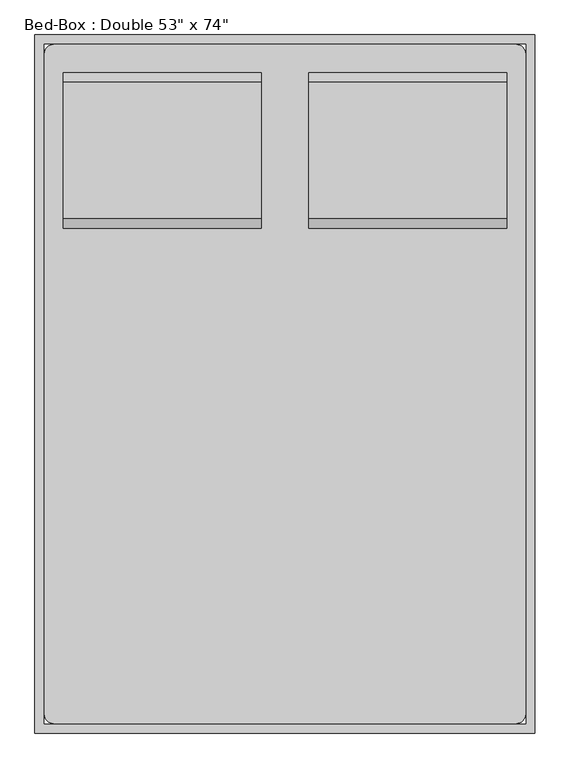
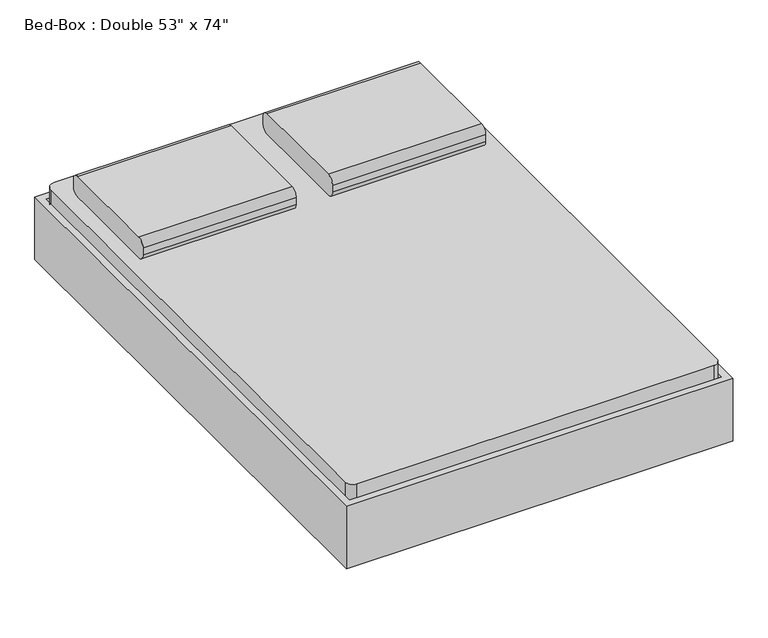
"""IFC4 building model written with IfcOpenShell, lengths in millimetres: furniture geometry."""

from ifc_helpers import new_model, si_unit, point, frame, frame_2d, origin, place, context, project, spatial, polyline, circle_curve, trimmed, segment, composite_curve, outline, extrude, source, transform, mapped, element, save
from ifc_brep_helpers import plane_surface, cylinder_surface, revolved_surface, advanced_brep


def furniture_c8abb964(model_context):
    return source(origin(), model_context, "Body", "SolidModel", [
        extrude(outline(composite_curve([segment(polyline([(578.3704918, 406.4), (210.0704918, 406.4)]), True, "CONTINUOUS"), segment(trimmed(circle_curve(frame_2d((210.0704918, 431.8)), 25.4), [point((210.0704918, 406.4))], [point((184.6704918, 431.8))], False, "CARTESIAN"), True, "CONTINUOUS"), segment(polyline([(184.6704918, 431.8), (184.6704918, 457.2)]), True, "CONTINUOUS"), segment(trimmed(circle_curve(frame_2d((210.0704918, 457.2)), 25.4), [point((184.6704918, 457.2))], [point((210.0704918, 482.6))], False, "CARTESIAN"), True, "CONTINUOUS"), segment(polyline([(210.0704918, 482.6), (578.3704918, 482.6)]), True, "CONTINUOUS"), segment(trimmed(circle_curve(frame_2d((578.3704918, 457.2)), 25.4), [point((578.3704918, 482.6))], [point((603.7704918, 457.2))], False, "CARTESIAN"), True, "CONTINUOUS"), segment(polyline([(603.7704918, 457.2), (603.7704918, 431.8)]), True, "CONTINUOUS"), segment(trimmed(circle_curve(frame_2d((578.3704918, 431.8)), 25.4), [point((603.7704918, 431.8))], [point((578.3704918, 406.4))], False, "CARTESIAN"), True, "CONTINUOUS")], self_intersect=False)), frame((402.652459, 0.0, 0.0), z_axis=(1.0, 0.0, 0.0), x_axis=(0.0, 1.0, 0.0)), (0.0, 0.0, 1.0), 533.4),
        extrude(outline(composite_curve([segment(polyline([(578.3704918, 406.4), (210.0704918, 406.4)]), True, "CONTINUOUS"), segment(trimmed(circle_curve(frame_2d((210.0704918, 431.8)), 25.4), [point((210.0704918, 406.4))], [point((184.6704918, 431.8))], False, "CARTESIAN"), True, "CONTINUOUS"), segment(polyline([(184.6704918, 431.8), (184.6704918, 457.2)]), True, "CONTINUOUS"), segment(trimmed(circle_curve(frame_2d((210.0704918, 457.2)), 25.4), [point((184.6704918, 457.2))], [point((210.0704918, 482.6))], False, "CARTESIAN"), True, "CONTINUOUS"), segment(polyline([(210.0704918, 482.6), (578.3704918, 482.6)]), True, "CONTINUOUS"), segment(trimmed(circle_curve(frame_2d((578.3704918, 457.2)), 25.4), [point((578.3704918, 482.6))], [point((603.7704918, 457.2))], False, "CARTESIAN"), True, "CONTINUOUS"), segment(polyline([(603.7704918, 457.2), (603.7704918, 431.8)]), True, "CONTINUOUS"), segment(trimmed(circle_curve(frame_2d((578.3704918, 431.8)), 25.4), [point((603.7704918, 431.8))], [point((578.3704918, 406.4))], False, "CARTESIAN"), True, "CONTINUOUS")], self_intersect=False)), frame((-257.747541, 0.0, 0.0), z_axis=(1.0, 0.0, 0.0), x_axis=(0.0, 1.0, 0.0)), (0.0, 0.0, 1.0), 533.4),
        advanced_brep(
        [(-308.2231784, 451.3704918, 177.8), (-308.2231784, 375.1704918, 177.8), (-308.2231784, 375.1704918, 196.85), (-308.2231784, 451.3704918, 196.85), (-257.4231784, 451.3704918, 177.8), (-257.4231784, 375.1704918, 177.8), (-245.2869899, 375.1704918, 196.85), (-245.2869899, 451.3704918, 196.85), (-181.3523099, 451.3704918, 14.6654962), (-181.3523099, 375.1704918, 14.6654962), (-164.0871466, 375.1704918, 22.716374), (-164.0871466, 451.3704918, 22.716374), (-158.3320921, 375.1704918, 0.0), (-158.3320921, 451.3704918, 0.0), (-158.3320921, 375.1704918, 19.05), (-158.3320921, 451.3704918, 19.05), (-79.7195862, 451.3704918, 0.0), (-79.7195862, 375.1704918, 0.0), (-79.7195862, 375.1704918, 19.05), (-79.7195862, 451.3704918, 19.05), (-67.0195862, 375.1704918, 3.4029547), (-67.0195862, 451.3704918, 3.4029547), (-76.5445862, 375.1704918, 19.9007387), (-76.5445862, 451.3704918, 19.9007387), (-6.922541, 451.3704918, 38.1), (-6.922541, 375.1704918, 38.1), (-12.0269731, 375.1704918, 57.15), (-12.0269731, 451.3704918, 57.15), (685.5518216, 451.3704918, 38.1), (685.5518216, 375.1704918, 38.1), (690.6562537, 375.1704918, 57.15), (690.6562537, 451.3704918, 57.15), (745.6488669, 451.3704918, 3.4029547), (745.6488669, 375.1704918, 3.4029547), (755.1738669, 375.1704918, 19.9007387), (755.1738669, 451.3704918, 19.9007387), (758.3488669, 375.1704918, 0.0), (758.3488669, 451.3704918, 0.0), (758.3488669, 375.1704918, 19.05), (758.3488669, 451.3704918, 19.05), (836.9613728, 451.3704918, 0.0), (836.9613728, 375.1704918, 0.0), (836.9613728, 375.1704918, 19.05), (836.9613728, 451.3704918, 19.05), (859.9815906, 375.1704918, 14.6654962), (859.9815906, 451.3704918, 14.6654962), (842.7164272, 375.1704918, 22.716374), (842.7164272, 451.3704918, 22.716374), (936.052459, 451.3704918, 177.8), (936.052459, 375.1704918, 177.8), (923.9162705, 375.1704918, 196.85), (923.9162705, 451.3704918, 196.85), (986.852459, 451.3704918, 177.8), (986.852459, 451.3704918, 196.85), (986.852459, 375.1704918, 196.85), (986.852459, 375.1704918, 177.8)],
        [
            (0, 1),
            (1, 2),
            (2, 3),
            (3, 0),
            (0, 4),
            (4, 5),
            (5, 1),
            (5, 6),
            (6, 2),
            (6, 7),
            (7, 3),
            (7, 4),
            (4, 8),
            (8, 9),
            (9, 5),
            (9, 10),
            (10, 6),
            (10, 11),
            (11, 7),
            (11, 8),
            (12, 9, circle_curve(frame((-158.3320921, 375.1704918, 25.4), z_axis=(0.0, 1.0, 0.0), x_axis=(-0.9063077870366486, 0.0, -0.42261826174070233)), 25.4)),
            (8, 13, circle_curve(frame((-158.3320921, 451.3704918, 25.4), z_axis=(0.0, -1.0, 0.0), x_axis=(-0.9063077870366486, 0.0, -0.42261826174070233)), 25.4)),
            (13, 12),
            (14, 10, circle_curve(frame((-158.3320921, 375.1704918, 25.4), z_axis=(0.0, 1.0, 0.0), x_axis=(-0.9063077870366486, 0.0, -0.42261826174070233)), 6.35)),
            (12, 14),
            (15, 11, circle_curve(frame((-158.3320921, 451.3704918, 25.4), z_axis=(0.0, 1.0, 0.0), x_axis=(-0.9063077870366486, 0.0, -0.42261826174070233)), 6.35)),
            (14, 15),
            (15, 13),
            (13, 16),
            (16, 17),
            (17, 12),
            (17, 18),
            (18, 14),
            (18, 19),
            (19, 15),
            (19, 16),
            (20, 17, circle_curve(frame((-79.7195862, 375.1704918, 25.4), z_axis=(0.0, 1.0, 0.0), x_axis=(0.0, 0.0, -1.0)), 25.4)),
            (16, 21, circle_curve(frame((-79.7195862, 451.3704918, 25.4), z_axis=(0.0, -1.0, 0.0), x_axis=(0.0, 0.0, -1.0)), 25.4)),
            (21, 20),
            (22, 18, circle_curve(frame((-79.7195862, 375.1704918, 25.4), z_axis=(0.0, 1.0, 0.0), x_axis=(0.0, 0.0, -1.0)), 6.35)),
            (20, 22),
            (23, 19, circle_curve(frame((-79.7195862, 451.3704918, 25.4), z_axis=(0.0, 1.0, 0.0), x_axis=(0.0, 0.0, -1.0)), 6.35)),
            (22, 23),
            (23, 21),
            (21, 24),
            (24, 25),
            (25, 20),
            (25, 26),
            (26, 22),
            (26, 27),
            (27, 23),
            (27, 24),
            (24, 28),
            (28, 29),
            (29, 25),
            (29, 30),
            (30, 26),
            (30, 31),
            (31, 27),
            (31, 28),
            (28, 32),
            (32, 33),
            (33, 29),
            (33, 34),
            (34, 30),
            (34, 35),
            (35, 31),
            (35, 32),
            (36, 33, circle_curve(frame((758.3488669, 375.1704918, 25.4), z_axis=(0.0, 1.0, 0.0), x_axis=(-0.5000000000000463, 0.0, -0.8660254037844118)), 25.4)),
            (32, 37, circle_curve(frame((758.3488669, 451.3704918, 25.4), z_axis=(0.0, -1.0, 0.0), x_axis=(-0.5000000000000463, 0.0, -0.8660254037844118)), 25.4)),
            (37, 36),
            (38, 34, circle_curve(frame((758.3488669, 375.1704918, 25.4), z_axis=(0.0, 1.0, 0.0), x_axis=(-0.5000000000000463, 0.0, -0.8660254037844118)), 6.35)),
            (36, 38),
            (39, 35, circle_curve(frame((758.3488669, 451.3704918, 25.4), z_axis=(0.0, 1.0, 0.0), x_axis=(-0.5000000000000463, 0.0, -0.8660254037844118)), 6.35)),
            (38, 39),
            (39, 37),
            (37, 40),
            (40, 41),
            (41, 36),
            (41, 42),
            (42, 38),
            (42, 43),
            (43, 39),
            (43, 40),
            (44, 41, circle_curve(frame((836.9613728, 375.1704918, 25.4), z_axis=(0.0, 1.0, 0.0), x_axis=(0.0, 0.0, -1.0)), 25.4)),
            (40, 45, circle_curve(frame((836.9613728, 451.3704918, 25.4), z_axis=(0.0, -1.0, 0.0), x_axis=(0.0, 0.0, -1.0)), 25.4)),
            (45, 44),
            (46, 42, circle_curve(frame((836.9613728, 375.1704918, 25.4), z_axis=(0.0, 1.0, 0.0), x_axis=(0.0, 0.0, -1.0)), 6.35)),
            (44, 46),
            (47, 43, circle_curve(frame((836.9613728, 451.3704918, 25.4), z_axis=(0.0, 1.0, 0.0), x_axis=(0.0, 0.0, -1.0)), 6.35)),
            (46, 47),
            (47, 45),
            (45, 48),
            (48, 49),
            (49, 44),
            (49, 50),
            (50, 46),
            (50, 51),
            (51, 47),
            (51, 48),
            (52, 53),
            (53, 54),
            (54, 55),
            (55, 52),
            (48, 52),
            (55, 49),
            (54, 50),
            (53, 51),
        ],
        [
            plane_surface(frame((-308.2231784, 705.3704918, -152.9490627), z_axis=(-1.0, 0.0, 0.0), x_axis=(0.0, 1.0, 0.0))),
            plane_surface(frame((-308.2231784, 451.3704918, 177.8), z_axis=(0.0, 0.0, -1.0), x_axis=(1.0, 0.0, 0.0))),
            plane_surface(frame((-308.2231784, 375.1704918, 177.8), z_axis=(0.0, -1.0, 0.0), x_axis=(1.0, 0.0, 0.0))),
            plane_surface(frame((-308.2231784, 375.1704918, 196.85), z_axis=(0.0, 0.0, 1.0), x_axis=(1.0, 0.0, 0.0))),
            plane_surface(frame((-308.2231784, 451.3704918, 196.85), z_axis=(0.0, 1.0, 0.0), x_axis=(1.0, 0.0, 0.0))),
            plane_surface(frame((-257.4231784, 451.3704918, 177.8), z_axis=(-0.9063077870366488, 0.0, -0.42261826174070194), x_axis=(0.42261826174070194, 0.0, -0.9063077870366488))),
            plane_surface(frame((-257.4231784, 375.1704918, 177.8), z_axis=(0.0, -1.0, 0.0), x_axis=(0.42261826174070194, 0.0, -0.9063077870366488))),
            plane_surface(frame((-245.2869899, 375.1704918, 196.85), z_axis=(0.9063077870366487, 0.0, 0.4226182617407021), x_axis=(0.4226182617407021, 0.0, -0.9063077870366487))),
            plane_surface(frame((-245.2869899, 451.3704918, 196.85), z_axis=(0.0, 1.0, 0.0), x_axis=(0.4226182617407021, 0.0, -0.9063077870366487))),
            cylinder_surface(frame((-158.3320921, 705.3704918, 25.4), z_axis=(0.0, -1.0, 0.0), x_axis=(-0.9063077870366486, 0.0, -0.42261826174070233)), 25.4),
            plane_surface(frame((-158.3320921, 375.1704918, 25.4), z_axis=(0.0, -1.0, 0.0), x_axis=(-0.9063077870366486, 0.0, -0.42261826174070233))),
            revolved_surface(polyline([(-164.08714654768272, 375.1704918, 22.71637403794654), (-164.08714654768272, 451.3704918, 22.71637403794654)]), (-158.3320921, 705.3704918, 25.4), (0.0, -1.0, 0.0)),
            plane_surface(frame((-158.3320921, 451.3704918, 25.4), z_axis=(0.0, 1.0, 0.0), x_axis=(-0.9063077870366486, 0.0, -0.42261826174070233))),
            plane_surface(frame((-158.3320921, 451.3704918, 0.0), z_axis=(0.0, 0.0, -1.0), x_axis=(1.0, 0.0, 0.0))),
            plane_surface(frame((-158.3320921, 375.1704918, 0.0), z_axis=(0.0, -1.0, 0.0), x_axis=(1.0, 0.0, 0.0))),
            plane_surface(frame((-158.3320921, 375.1704918, 19.05), z_axis=(0.0, 0.0, 1.0), x_axis=(1.0, 0.0, 0.0))),
            plane_surface(frame((-158.3320921, 451.3704918, 19.05), z_axis=(0.0, 1.0, 0.0), x_axis=(1.0, 0.0, 0.0))),
            cylinder_surface(frame((-79.7195862, 705.3704918, 25.4), z_axis=(0.0, -1.0, 0.0), x_axis=(0.0, 0.0, -1.0)), 25.4),
            plane_surface(frame((-79.7195862, 375.1704918, 25.4), z_axis=(0.0, -1.0, 0.0), x_axis=(0.0, 0.0, -1.0))),
            revolved_surface(polyline([(-79.7195862, 375.1704918, 19.049999999999997), (-79.7195862, 451.3704918, 19.049999999999997)]), (-79.7195862, 705.3704918, 25.4), (0.0, -1.0, 0.0)),
            plane_surface(frame((-79.7195862, 451.3704918, 25.4), z_axis=(0.0, 1.0, 0.0), x_axis=(0.0, 0.0, -1.0))),
            plane_surface(frame((-67.0195862, 451.3704918, 3.4029547), z_axis=(0.4999999999998775, 0.0, -0.8660254037845094), x_axis=(0.8660254037845094, 0.0, 0.4999999999998775))),
            plane_surface(frame((-67.0195862, 375.1704918, 3.4029547), z_axis=(0.0, -1.0, 0.0), x_axis=(0.866025403784509, 0.0, 0.49999999999987826))),
            plane_surface(frame((-76.5445862, 375.1704918, 19.9007387), z_axis=(-0.49999999999987754, 0.0, 0.8660254037845093), x_axis=(0.8660254037845093, 0.0, 0.49999999999987754))),
            plane_surface(frame((-76.5445862, 451.3704918, 19.9007387), z_axis=(0.0, 1.0000000000000002, 0.0), x_axis=(0.8660254037845091, 0.0, 0.49999999999987815))),
            plane_surface(frame((-6.922541, 451.3704918, 38.1), z_axis=(0.0, 0.0, -1.0), x_axis=(1.0, 0.0, 0.0))),
            plane_surface(frame((-6.922541, 375.1704918, 38.1), z_axis=(0.0, -1.0, 0.0), x_axis=(1.0, 0.0, 0.0))),
            plane_surface(frame((-12.0269731, 375.1704918, 57.15), z_axis=(0.0, 0.0, 1.0), x_axis=(1.0, 0.0, 0.0))),
            plane_surface(frame((-12.0269731, 451.3704918, 57.15), z_axis=(0.0, 1.0, 0.0), x_axis=(1.0, 0.0, 0.0))),
            plane_surface(frame((685.5518216, 451.3704918, 38.1), z_axis=(-0.500000000000047, 0.0, -0.8660254037844116), x_axis=(0.8660254037844116, 0.0, -0.500000000000047))),
            plane_surface(frame((685.5518216, 375.1704918, 38.1), z_axis=(0.0, -1.0, 0.0), x_axis=(0.8660254037844122, 0.0, -0.5000000000000459))),
            plane_surface(frame((690.6562537, 375.1704918, 57.15), z_axis=(0.5000000000000461, 0.0, 0.8660254037844121), x_axis=(0.8660254037844121, 0.0, -0.5000000000000461))),
            plane_surface(frame((690.6562537, 451.3704918, 57.15), z_axis=(0.0, 1.0, 0.0), x_axis=(0.8660254037844127, 0.0, -0.500000000000045))),
            cylinder_surface(frame((758.3488669, 705.3704918, 25.4), z_axis=(0.0, -1.0, 0.0), x_axis=(-0.5000000000000463, 0.0, -0.8660254037844118)), 25.4),
            plane_surface(frame((758.3488669, 375.1704918, 25.4), z_axis=(0.0, -1.0000000000000002, 0.0), x_axis=(-0.5000000000000464, 0.0, -0.866025403784412))),
            revolved_surface(polyline([(755.1738668999997, 375.1704918, 19.90073868596898), (755.1738668999997, 451.3704918, 19.90073868596898)]), (758.3488669, 705.3704918, 25.4), (0.0, -1.0, 0.0)),
            plane_surface(frame((758.3488669, 451.3704918, 25.4), z_axis=(0.0, 1.0000000000000002, 0.0), x_axis=(-0.5000000000000464, 0.0, -0.866025403784412))),
            plane_surface(frame((758.3488669, 451.3704918, 0.0), z_axis=(0.0, 0.0, -1.0), x_axis=(1.0, 0.0, 0.0))),
            plane_surface(frame((758.3488669, 375.1704918, 0.0), z_axis=(0.0, -1.0, 0.0), x_axis=(1.0, 0.0, 0.0))),
            plane_surface(frame((758.3488669, 375.1704918, 19.05), z_axis=(0.0, 0.0, 1.0), x_axis=(1.0, 0.0, 0.0))),
            plane_surface(frame((758.3488669, 451.3704918, 19.05), z_axis=(0.0, 1.0, 0.0), x_axis=(1.0, 0.0, 0.0))),
            cylinder_surface(frame((836.9613728, 705.3704918, 25.4), z_axis=(0.0, -1.0, 0.0), x_axis=(0.0, 0.0, -1.0)), 25.4),
            plane_surface(frame((836.9613728, 375.1704918, 25.4), z_axis=(0.0, -1.0, 0.0), x_axis=(0.0, 0.0, -1.0))),
            revolved_surface(polyline([(836.9613728, 375.1704918, 19.049999999999997), (836.9613728, 451.3704918, 19.049999999999997)]), (836.9613728, 705.3704918, 25.4), (0.0, -1.0, 0.0)),
            plane_surface(frame((836.9613728, 451.3704918, 25.4), z_axis=(0.0, 1.0, 0.0), x_axis=(0.0, 0.0, -1.0))),
            plane_surface(frame((859.9815906, 451.3704918, 14.6654962), z_axis=(0.9063077870366797, 0.0, -0.42261826174063566), x_axis=(0.42261826174063566, 0.0, 0.9063077870366797))),
            plane_surface(frame((859.9815906, 375.1704918, 14.6654962), z_axis=(0.0, -1.0000000000000002, 0.0), x_axis=(0.4226182617406349, 0.0, 0.9063077870366801))),
            plane_surface(frame((842.7164272, 375.1704918, 22.716374), z_axis=(-0.9063077870366799, 0.0, 0.4226182617406354), x_axis=(0.4226182617406354, 0.0, 0.9063077870366799))),
            plane_surface(frame((842.7164272, 451.3704918, 22.716374), z_axis=(0.0, 1.0, 0.0), x_axis=(0.42261826174063555, 0.0, 0.9063077870366798))),
            plane_surface(frame((986.852459, 705.3704918, -152.9490627), z_axis=(1.0, 0.0, 0.0), x_axis=(0.0, 1.0, 0.0))),
            plane_surface(frame((936.052459, 451.3704918, 177.8), z_axis=(0.0, 0.0, -1.0), x_axis=(1.0, 0.0, 0.0))),
            plane_surface(frame((936.052459, 375.1704918, 177.8), z_axis=(0.0, -1.0, 0.0), x_axis=(1.0, 0.0, 0.0))),
            plane_surface(frame((923.9162705, 375.1704918, 196.85), z_axis=(0.0, 0.0, 1.0), x_axis=(1.0, 0.0, 0.0))),
            plane_surface(frame((923.9162705, 451.3704918, 196.85), z_axis=(0.0, 1.0, 0.0), x_axis=(1.0, 0.0, 0.0))),
        ],
        [
            (0, [[1, 2, 3, 4]]),
            (1, [[-1, 5, 6, 7]]),
            (2, [[-2, -7, 8, 9]]),
            (3, [[-3, -9, 10, 11]]),
            (4, [[-4, -11, 12, -5]]),
            (5, [[-6, 13, 14, 15]]),
            (6, [[-8, -15, 16, 17]]),
            (7, [[-10, -17, 18, 19]]),
            (8, [[-12, -19, 20, -13]]),
            (9, [[21, -14, 22, 23]]),
            (10, [[24, -16, -21, 25]]),
            (11, [[26, -18, -24, 27]]),
            (12, [[-22, -20, -26, 28]]),
            (13, [[-23, 29, 30, 31]]),
            (14, [[-25, -31, 32, 33]]),
            (15, [[-27, -33, 34, 35]]),
            (16, [[-28, -35, 36, -29]]),
            (17, [[37, -30, 38, 39]]),
            (18, [[40, -32, -37, 41]]),
            (19, [[42, -34, -40, 43]]),
            (20, [[-38, -36, -42, 44]]),
            (21, [[-39, 45, 46, 47]]),
            (22, [[-41, -47, 48, 49]]),
            (23, [[-43, -49, 50, 51]]),
            (24, [[-44, -51, 52, -45]]),
            (25, [[-46, 53, 54, 55]]),
            (26, [[-48, -55, 56, 57]]),
            (27, [[-50, -57, 58, 59]]),
            (28, [[-52, -59, 60, -53]]),
            (29, [[-54, 61, 62, 63]]),
            (30, [[-56, -63, 64, 65]]),
            (31, [[-58, -65, 66, 67]]),
            (32, [[-60, -67, 68, -61]]),
            (33, [[69, -62, 70, 71]]),
            (34, [[72, -64, -69, 73]]),
            (35, [[74, -66, -72, 75]]),
            (36, [[-70, -68, -74, 76]]),
            (37, [[-71, 77, 78, 79]]),
            (38, [[-73, -79, 80, 81]]),
            (39, [[-75, -81, 82, 83]]),
            (40, [[-76, -83, 84, -77]]),
            (41, [[85, -78, 86, 87]]),
            (42, [[88, -80, -85, 89]]),
            (43, [[90, -82, -88, 91]]),
            (44, [[-86, -84, -90, 92]]),
            (45, [[-87, 93, 94, 95]]),
            (46, [[-89, -95, 96, 97]]),
            (47, [[-91, -97, 98, 99]]),
            (48, [[-92, -99, 100, -93]]),
            (49, [[101, 102, 103, 104]]),
            (50, [[-94, 105, -104, 106]]),
            (51, [[-96, -106, -103, 107]]),
            (52, [[-98, -107, -102, 108]]),
            (53, [[-100, -108, -101, -105]]),
        ],
    ),
        extrude(outline(composite_curve([segment(polyline([(-283.147541, 679.9704918), (961.452459, 679.9704918)]), True, "CONTINUOUS"), segment(trimmed(circle_curve(frame_2d((961.452459, 654.5704918)), 25.4), [point((961.452459, 679.9704918))], [point((986.852459, 654.5704918))], False, "CARTESIAN"), True, "CONTINUOUS"), segment(polyline([(986.852459, 654.5704918), (986.852459, -1123.4295082)]), True, "CONTINUOUS"), segment(trimmed(circle_curve(frame_2d((961.452459, -1123.4295082)), 25.4), [point((986.852459, -1123.4295082))], [point((961.452459, -1148.8295082))], False, "CARTESIAN"), True, "CONTINUOUS"), segment(polyline([(961.452459, -1148.8295082), (-283.147541, -1148.8295082)]), True, "CONTINUOUS"), segment(trimmed(circle_curve(frame_2d((-283.147541, -1123.4295082)), 25.4), [point((-283.147541, -1148.8295082))], [point((-308.547541, -1123.4295082))], False, "CARTESIAN"), True, "CONTINUOUS"), segment(polyline([(-308.547541, -1123.4295082), (-308.547541, 654.5704918)]), True, "CONTINUOUS"), segment(trimmed(circle_curve(frame_2d((-283.147541, 654.5704918)), 25.4), [point((-308.547541, 654.5704918))], [point((-283.147541, 679.9704918))], False, "CARTESIAN"), True, "CONTINUOUS")], self_intersect=False)), frame((0.0, 0.0, 203.2), z_axis=(0.0, 0.0, 1.0), x_axis=(1.0, 0.0, 0.0)), (0.0, 0.0, 1.0), 203.2),
        advanced_brep(
        [(-308.547541, -869.4295082, 196.85), (-308.547541, -869.4295082, 177.8), (-308.547541, -945.6295082, 177.8), (-308.547541, -945.6295082, 196.85), (-245.6113525, -869.4295082, 196.85), (-257.747541, -869.4295082, 177.8), (-257.747541, -945.6295082, 177.8), (-245.6113525, -945.6295082, 196.85), (-164.4115092, -869.4295082, 22.716374), (-181.6766725, -869.4295082, 14.6654962), (-181.6766725, -945.6295082, 14.6654962), (-164.4115092, -945.6295082, 22.716374), (-158.6564547, -869.4295082, 0.0), (-158.6564547, -869.4295082, 19.05), (-158.6564547, -945.6295082, 0.0), (-158.6564547, -945.6295082, 19.05), (-80.0439489, -869.4295082, 19.05), (-80.0439489, -869.4295082, 0.0), (-80.0439489, -945.6295082, 0.0), (-80.0439489, -945.6295082, 19.05), (-67.3439489, -869.4295082, 3.4029547), (-76.8689489, -869.4295082, 19.9007387), (-67.3439489, -945.6295082, 3.4029547), (-76.8689489, -945.6295082, 19.9007387), (-12.3513357, -869.4295082, 57.15), (-7.2469036, -869.4295082, 38.1), (-7.2469036, -945.6295082, 38.1), (-12.3513357, -945.6295082, 57.15), (690.6562537, -869.4295082, 57.15), (685.5518216, -869.4295082, 38.1), (685.5518216, -945.6295082, 38.1), (690.6562537, -945.6295082, 57.15), (755.1738669, -869.4295082, 19.9007387), (745.6488669, -869.4295082, 3.4029547), (745.6488669, -945.6295082, 3.4029547), (755.1738669, -945.6295082, 19.9007387), (758.3488669, -869.4295082, 0.0), (758.3488669, -869.4295082, 19.05), (758.3488669, -945.6295082, 0.0), (758.3488669, -945.6295082, 19.05), (836.9613728, -869.4295082, 19.05), (836.9613728, -869.4295082, 0.0), (836.9613728, -945.6295082, 0.0), (836.9613728, -945.6295082, 19.05), (859.9815906, -869.4295082, 14.6654962), (842.7164272, -869.4295082, 22.716374), (859.9815906, -945.6295082, 14.6654962), (842.7164272, -945.6295082, 22.716374), (923.9162705, -869.4295082, 196.85), (936.052459, -869.4295082, 177.8), (936.052459, -945.6295082, 177.8), (923.9162705, -945.6295082, 196.85), (986.852459, -869.4295082, 196.85), (986.852459, -945.6295082, 196.85), (986.852459, -945.6295082, 177.8), (986.852459, -869.4295082, 177.8)],
        [
            (0, 1),
            (1, 2),
            (2, 3),
            (3, 0),
            (0, 4),
            (4, 5),
            (5, 1),
            (5, 6),
            (6, 2),
            (6, 7),
            (7, 3),
            (7, 4),
            (4, 8),
            (8, 9),
            (9, 5),
            (9, 10),
            (10, 6),
            (10, 11),
            (11, 7),
            (11, 8),
            (12, 9, circle_curve(frame((-158.6564547, -869.4295082, 25.4), z_axis=(0.0, 1.0, 0.0), x_axis=(-0.906307787036663, 0.0, -0.4226182617406713)), 25.4)),
            (8, 13, circle_curve(frame((-158.6564547, -869.4295082, 25.4), z_axis=(0.0, -1.0, 0.0), x_axis=(-0.906307787036663, 0.0, -0.4226182617406713)), 6.35)),
            (13, 12),
            (14, 10, circle_curve(frame((-158.6564547, -945.6295082, 25.4), z_axis=(0.0, 1.0, 0.0), x_axis=(-0.906307787036663, 0.0, -0.4226182617406713)), 25.4)),
            (12, 14),
            (15, 11, circle_curve(frame((-158.6564547, -945.6295082, 25.4), z_axis=(0.0, 1.0, 0.0), x_axis=(-0.906307787036663, 0.0, -0.4226182617406713)), 6.35)),
            (14, 15),
            (15, 13),
            (13, 16),
            (16, 17),
            (17, 12),
            (17, 18),
            (18, 14),
            (18, 19),
            (19, 15),
            (19, 16),
            (20, 17, circle_curve(frame((-80.0439489, -869.4295082, 25.4), z_axis=(0.0, 1.0, 0.0), x_axis=(0.0, 0.0, -1.0)), 25.4)),
            (16, 21, circle_curve(frame((-80.0439489, -869.4295082, 25.4), z_axis=(0.0, -1.0, 0.0), x_axis=(0.0, 0.0, -1.0)), 6.35)),
            (21, 20),
            (22, 18, circle_curve(frame((-80.0439489, -945.6295082, 25.4), z_axis=(0.0, 1.0, 0.0), x_axis=(0.0, 0.0, -1.0)), 25.4)),
            (20, 22),
            (23, 19, circle_curve(frame((-80.0439489, -945.6295082, 25.4), z_axis=(0.0, 1.0, 0.0), x_axis=(0.0, 0.0, -1.0)), 6.35)),
            (22, 23),
            (23, 21),
            (21, 24),
            (24, 25),
            (25, 20),
            (25, 26),
            (26, 22),
            (26, 27),
            (27, 23),
            (27, 24),
            (24, 28),
            (28, 29),
            (29, 25),
            (29, 30),
            (30, 26),
            (30, 31),
            (31, 27),
            (31, 28),
            (28, 32),
            (32, 33),
            (33, 29),
            (33, 34),
            (34, 30),
            (34, 35),
            (35, 31),
            (35, 32),
            (36, 33, circle_curve(frame((758.3488669, -869.4295082, 25.4), z_axis=(0.0, 1.0, 0.0), x_axis=(-0.5000000000000479, 0.0, -0.866025403784411)), 25.4)),
            (32, 37, circle_curve(frame((758.3488669, -869.4295082, 25.4), z_axis=(0.0, -1.0, 0.0), x_axis=(-0.5000000000000479, 0.0, -0.866025403784411)), 6.35)),
            (37, 36),
            (38, 34, circle_curve(frame((758.3488669, -945.6295082, 25.4), z_axis=(0.0, 1.0, 0.0), x_axis=(-0.5000000000000479, 0.0, -0.866025403784411)), 25.4)),
            (36, 38),
            (39, 35, circle_curve(frame((758.3488669, -945.6295082, 25.4), z_axis=(0.0, 1.0, 0.0), x_axis=(-0.5000000000000479, 0.0, -0.866025403784411)), 6.35)),
            (38, 39),
            (39, 37),
            (37, 40),
            (40, 41),
            (41, 36),
            (41, 42),
            (42, 38),
            (42, 43),
            (43, 39),
            (43, 40),
            (44, 41, circle_curve(frame((836.9613728, -869.4295082, 25.4), z_axis=(0.0, 1.0, 0.0), x_axis=(0.0, 0.0, -1.0)), 25.4)),
            (40, 45, circle_curve(frame((836.9613728, -869.4295082, 25.4), z_axis=(0.0, -1.0, 0.0), x_axis=(0.0, 0.0, -1.0)), 6.35)),
            (45, 44),
            (46, 42, circle_curve(frame((836.9613728, -945.6295082, 25.4), z_axis=(0.0, 1.0, 0.0), x_axis=(0.0, 0.0, -1.0)), 25.4)),
            (44, 46),
            (47, 43, circle_curve(frame((836.9613728, -945.6295082, 25.4), z_axis=(0.0, 1.0, 0.0), x_axis=(0.0, 0.0, -1.0)), 6.35)),
            (46, 47),
            (47, 45),
            (45, 48),
            (48, 49),
            (49, 44),
            (49, 50),
            (50, 46),
            (50, 51),
            (51, 47),
            (51, 48),
            (52, 53),
            (53, 54),
            (54, 55),
            (55, 52),
            (48, 52),
            (55, 49),
            (54, 50),
            (53, 51),
        ],
        [
            plane_surface(frame((-308.547541, -1174.2295082, -127.5947323), z_axis=(-1.0, 0.0, 0.0), x_axis=(0.0, 1.0, 0.0))),
            plane_surface(frame((-308.547541, -869.4295082, 196.85), z_axis=(0.0, 1.0, 0.0), x_axis=(1.0, 0.0, 0.0))),
            plane_surface(frame((-308.547541, -869.4295082, 177.8), z_axis=(0.0, 0.0, -1.0), x_axis=(1.0, 0.0, 0.0))),
            plane_surface(frame((-308.547541, -945.6295082, 177.8), z_axis=(0.0, -1.0, 0.0), x_axis=(1.0, 0.0, 0.0))),
            plane_surface(frame((-308.547541, -945.6295082, 196.85), z_axis=(0.0, 0.0, 1.0), x_axis=(1.0, 0.0, 0.0))),
            plane_surface(frame((-245.6113525, -869.4295082, 196.85), z_axis=(0.0, 1.0, 0.0), x_axis=(0.422618261740671, 0.0, -0.9063077870366633))),
            plane_surface(frame((-257.747541, -869.4295082, 177.8), z_axis=(-0.9063077870366631, 0.0, -0.42261826174067113), x_axis=(0.42261826174067113, 0.0, -0.9063077870366631))),
            plane_surface(frame((-257.747541, -945.6295082, 177.8), z_axis=(0.0, -1.0, 0.0), x_axis=(0.42261826174067135, 0.0, -0.906307787036663))),
            plane_surface(frame((-245.6113525, -945.6295082, 196.85), z_axis=(0.9063077870366631, 0.0, 0.4226182617406713), x_axis=(0.4226182617406713, 0.0, -0.9063077870366631))),
            plane_surface(frame((-158.6564547, -869.4295082, 25.4), z_axis=(0.0, 1.0, 0.0), x_axis=(-0.906307787036663, 0.0, -0.4226182617406713))),
            cylinder_surface(frame((-158.6564547, -1174.2295082, 25.4), z_axis=(0.0, -1.0, 0.0), x_axis=(-0.906307787036663, 0.0, -0.4226182617406713)), 25.4),
            plane_surface(frame((-158.6564547, -945.6295082, 25.4), z_axis=(0.0, -1.0, 0.0), x_axis=(-0.906307787036663, 0.0, -0.4226182617406713))),
            revolved_surface(polyline([(-164.41150914768284, -945.6295082, 22.716374037946736), (-164.41150914768284, -869.4295082, 22.716374037946736)]), (-158.6564547, -1174.2295082, 25.4), (0.0, -1.0, 0.0)),
            plane_surface(frame((-158.6564547, -869.4295082, 19.05), z_axis=(0.0, 1.0, 0.0), x_axis=(1.0, 0.0, 0.0))),
            plane_surface(frame((-158.6564547, -869.4295082, 0.0), z_axis=(0.0, 0.0, -1.0), x_axis=(1.0, 0.0, 0.0))),
            plane_surface(frame((-158.6564547, -945.6295082, 0.0), z_axis=(0.0, -1.0, 0.0), x_axis=(1.0, 0.0, 0.0))),
            plane_surface(frame((-158.6564547, -945.6295082, 19.05), z_axis=(0.0, 0.0, 1.0), x_axis=(1.0, 0.0, 0.0))),
            plane_surface(frame((-80.0439489, -869.4295082, 25.4), z_axis=(0.0, 1.0, 0.0), x_axis=(0.0, 0.0, -1.0))),
            cylinder_surface(frame((-80.0439489, -1174.2295082, 25.4), z_axis=(0.0, -1.0, 0.0), x_axis=(0.0, 0.0, -1.0)), 25.4),
            plane_surface(frame((-80.0439489, -945.6295082, 25.4), z_axis=(0.0, -1.0, 0.0), x_axis=(0.0, 0.0, -1.0))),
            revolved_surface(polyline([(-80.0439489, -945.6295082, 19.049999999999997), (-80.0439489, -869.4295082, 19.049999999999997)]), (-80.0439489, -1174.2295082, 25.4), (0.0, -1.0, 0.0)),
            plane_surface(frame((-76.8689489, -869.4295082, 19.9007387), z_axis=(0.0, 1.0, 0.0), x_axis=(0.8660254037844785, 0.0, 0.499999999999931))),
            plane_surface(frame((-67.3439489, -869.4295082, 3.4029547), z_axis=(0.499999999999931, 0.0, -0.8660254037844785), x_axis=(0.8660254037844785, 0.0, 0.499999999999931))),
            plane_surface(frame((-67.3439489, -945.6295082, 3.4029547), z_axis=(0.0, -1.0, 0.0), x_axis=(0.8660254037844786, 0.0, 0.49999999999993094))),
            plane_surface(frame((-76.8689489, -945.6295082, 19.9007387), z_axis=(-0.4999999999999312, 0.0, 0.8660254037844785), x_axis=(0.8660254037844785, 0.0, 0.4999999999999312))),
            plane_surface(frame((-12.3513357, -869.4295082, 57.15), z_axis=(0.0, 1.0, 0.0), x_axis=(1.0, 0.0, 0.0))),
            plane_surface(frame((-7.2469036, -869.4295082, 38.1), z_axis=(0.0, 0.0, -1.0), x_axis=(1.0, 0.0, 0.0))),
            plane_surface(frame((-7.2469036, -945.6295082, 38.1), z_axis=(0.0, -1.0, 0.0), x_axis=(1.0, 0.0, 0.0))),
            plane_surface(frame((-12.3513357, -945.6295082, 57.15), z_axis=(0.0, 0.0, 1.0), x_axis=(1.0, 0.0, 0.0))),
            plane_surface(frame((690.6562537, -869.4295082, 57.15), z_axis=(0.0, 1.0, 0.0), x_axis=(0.8660254037844091, 0.0, -0.5000000000000514))),
            plane_surface(frame((685.5518216, -869.4295082, 38.1), z_axis=(-0.5000000000000502, 0.0, -0.8660254037844097), x_axis=(0.8660254037844097, 0.0, -0.5000000000000502))),
            plane_surface(frame((685.5518216, -945.6295082, 38.1), z_axis=(0.0, -1.0, 0.0), x_axis=(0.86602540378441, 0.0, -0.5000000000000498))),
            plane_surface(frame((690.6562537, -945.6295082, 57.15), z_axis=(0.5000000000000505, 0.0, 0.8660254037844095), x_axis=(0.8660254037844095, 0.0, -0.5000000000000505))),
            plane_surface(frame((758.3488669, -869.4295082, 25.4), z_axis=(0.0, 1.0000000000000002, 0.0), x_axis=(-0.500000000000048, 0.0, -0.8660254037844111))),
            cylinder_surface(frame((758.3488669, -1174.2295082, 25.4), z_axis=(0.0, -1.0, 0.0), x_axis=(-0.5000000000000479, 0.0, -0.866025403784411)), 25.4),
            plane_surface(frame((758.3488669, -945.6295082, 25.4), z_axis=(0.0, -1.0000000000000002, 0.0), x_axis=(-0.500000000000048, 0.0, -0.8660254037844111))),
            revolved_surface(polyline([(755.1738668999997, -945.6295082, 19.90073868596899), (755.1738668999997, -869.4295082, 19.90073868596899)]), (758.3488669, -1174.2295082, 25.4), (0.0, -1.0, 0.0)),
            plane_surface(frame((758.3488669, -869.4295082, 19.05), z_axis=(0.0, 1.0, 0.0), x_axis=(1.0, 0.0, 0.0))),
            plane_surface(frame((758.3488669, -869.4295082, 0.0), z_axis=(0.0, 0.0, -1.0), x_axis=(1.0, 0.0, 0.0))),
            plane_surface(frame((758.3488669, -945.6295082, 0.0), z_axis=(0.0, -1.0, 0.0), x_axis=(1.0, 0.0, 0.0))),
            plane_surface(frame((758.3488669, -945.6295082, 19.05), z_axis=(0.0, 0.0, 1.0), x_axis=(1.0, 0.0, 0.0))),
            plane_surface(frame((836.9613728, -869.4295082, 25.4), z_axis=(0.0, 1.0, 0.0), x_axis=(0.0, 0.0, -1.0))),
            cylinder_surface(frame((836.9613728, -1174.2295082, 25.4), z_axis=(0.0, -1.0, 0.0), x_axis=(0.0, 0.0, -1.0)), 25.4),
            plane_surface(frame((836.9613728, -945.6295082, 25.4), z_axis=(0.0, -1.0, 0.0), x_axis=(0.0, 0.0, -1.0))),
            revolved_surface(polyline([(836.9613728, -945.6295082, 19.049999999999997), (836.9613728, -869.4295082, 19.049999999999997)]), (836.9613728, -1174.2295082, 25.4), (0.0, -1.0, 0.0)),
            plane_surface(frame((842.7164272, -869.4295082, 22.716374), z_axis=(0.0, 1.0, 0.0), x_axis=(0.4226182617405411, 0.0, 0.9063077870367238))),
            plane_surface(frame((859.9815906, -869.4295082, 14.6654962), z_axis=(0.9063077870367237, 0.0, -0.42261826174054157), x_axis=(0.42261826174054157, 0.0, 0.9063077870367237))),
            plane_surface(frame((859.9815906, -945.6295082, 14.6654962), z_axis=(0.0, -1.0, 0.0), x_axis=(0.4226182617405412, 0.0, 0.9063077870367238))),
            plane_surface(frame((842.7164272, -945.6295082, 22.716374), z_axis=(-0.906307787036724, 0.0, 0.422618261740541), x_axis=(0.422618261740541, 0.0, 0.906307787036724))),
            plane_surface(frame((986.852459, -1174.2295082, -127.5947323), z_axis=(1.0, 0.0, 0.0), x_axis=(0.0, 1.0, 0.0))),
            plane_surface(frame((923.9162705, -869.4295082, 196.85), z_axis=(0.0, 1.0, 0.0), x_axis=(1.0, 0.0, 0.0))),
            plane_surface(frame((936.052459, -869.4295082, 177.8), z_axis=(0.0, 0.0, -1.0), x_axis=(1.0, 0.0, 0.0))),
            plane_surface(frame((936.052459, -945.6295082, 177.8), z_axis=(0.0, -1.0, 0.0), x_axis=(1.0, 0.0, 0.0))),
            plane_surface(frame((923.9162705, -945.6295082, 196.85), z_axis=(0.0, 0.0, 1.0), x_axis=(1.0, 0.0, 0.0))),
        ],
        [
            (0, [[1, 2, 3, 4]]),
            (1, [[-1, 5, 6, 7]]),
            (2, [[-2, -7, 8, 9]]),
            (3, [[-3, -9, 10, 11]]),
            (4, [[-4, -11, 12, -5]]),
            (5, [[-6, 13, 14, 15]]),
            (6, [[-8, -15, 16, 17]]),
            (7, [[-10, -17, 18, 19]]),
            (8, [[-12, -19, 20, -13]]),
            (9, [[21, -14, 22, 23]]),
            (10, [[24, -16, -21, 25]]),
            (11, [[26, -18, -24, 27]]),
            (12, [[-22, -20, -26, 28]]),
            (13, [[-23, 29, 30, 31]]),
            (14, [[-25, -31, 32, 33]]),
            (15, [[-27, -33, 34, 35]]),
            (16, [[-28, -35, 36, -29]]),
            (17, [[37, -30, 38, 39]]),
            (18, [[40, -32, -37, 41]]),
            (19, [[42, -34, -40, 43]]),
            (20, [[-38, -36, -42, 44]]),
            (21, [[-39, 45, 46, 47]]),
            (22, [[-41, -47, 48, 49]]),
            (23, [[-43, -49, 50, 51]]),
            (24, [[-44, -51, 52, -45]]),
            (25, [[-46, 53, 54, 55]]),
            (26, [[-48, -55, 56, 57]]),
            (27, [[-50, -57, 58, 59]]),
            (28, [[-52, -59, 60, -53]]),
            (29, [[-54, 61, 62, 63]]),
            (30, [[-56, -63, 64, 65]]),
            (31, [[-58, -65, 66, 67]]),
            (32, [[-60, -67, 68, -61]]),
            (33, [[69, -62, 70, 71]]),
            (34, [[72, -64, -69, 73]]),
            (35, [[74, -66, -72, 75]]),
            (36, [[-70, -68, -74, 76]]),
            (37, [[-71, 77, 78, 79]]),
            (38, [[-73, -79, 80, 81]]),
            (39, [[-75, -81, 82, 83]]),
            (40, [[-76, -83, 84, -77]]),
            (41, [[85, -78, 86, 87]]),
            (42, [[88, -80, -85, 89]]),
            (43, [[90, -82, -88, 91]]),
            (44, [[-86, -84, -90, 92]]),
            (45, [[-87, 93, 94, 95]]),
            (46, [[-89, -95, 96, 97]]),
            (47, [[-91, -97, 98, 99]]),
            (48, [[-92, -99, 100, -93]]),
            (49, [[101, 102, 103, 104]]),
            (50, [[-94, 105, -104, 106]]),
            (51, [[-96, -106, -103, 107]]),
            (52, [[-98, -107, -102, 108]]),
            (53, [[-100, -108, -101, -105]]),
        ],
    ),
        extrude(outline(polyline([(1012.252459, 705.3704918), (1012.252459, -1174.2295082), (-333.947541, -1174.2295082), (-333.947541, 705.3704918), (1012.252459, 705.3704918)]), holes=[polyline([(986.852459, 679.9704918), (-308.547541, 679.9704918), (-308.547541, -1148.8295082), (986.852459, -1148.8295082), (986.852459, 679.9704918)])]), frame((0.0, 0.0, 127.0), z_axis=(0.0, 0.0, 1.0), x_axis=(1.0, 0.0, 0.0)), (0.0, 0.0, 1.0), 228.6),
    ])


if __name__ == "__main__":
    model = new_model("IFC4")
    model_context = context("Model", 3, world=origin())
    ifc_project = project(units=[si_unit("LENGTHUNIT", "METRE", prefix="MILLI")], contexts=[model_context])
    site = spatial("IfcSite", under=ifc_project)
    building = spatial("IfcBuilding", under=site)
    placement = place(None, origin())
    furniture_shape = furniture_c8abb964(model_context)
    element("IfcFurniture", 1, ObjectType="Bed-Box : Double 53\" x 74\"", at=placement, inside=building, context=model_context, shape_type="MappedRepresentation", body=[
        mapped(furniture_shape, transform((0.0, 0.0, 0.0), x_axis=(1.0, 0.0, 0.0), y_axis=(0.0, 1.0, 0.0), z_axis=(0.0, 0.0, 1.0))),
    ])
    save(model, "model.ifc")

# Revit data of these elements
# Type "Bed-Box : Double 53\" x 74\""
#   Assembly Code = "E2020200"
#   Length = 6' - 2"
#   Width = 4' - 5"
#   Frame Material = Birch
#   Mattress Material = Linen, White
#   Default Elevation = 0
# Element 1 (IfcFurniture, "Bed-Box : Double 53\" x 74\"")
#   Materials on its faces: "Birch", "Linen, White"
# Materials
#   "Birch": class "Wood", colour RGB 224 178 126, transparency 0, Description = "Betula Alleghaniensis", Cost = 0
#   "Linen, White": class "Textile", colour RGB 247 247 239, transparency 0, Description = "Linen, white", Cost = 0
